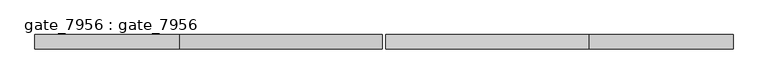
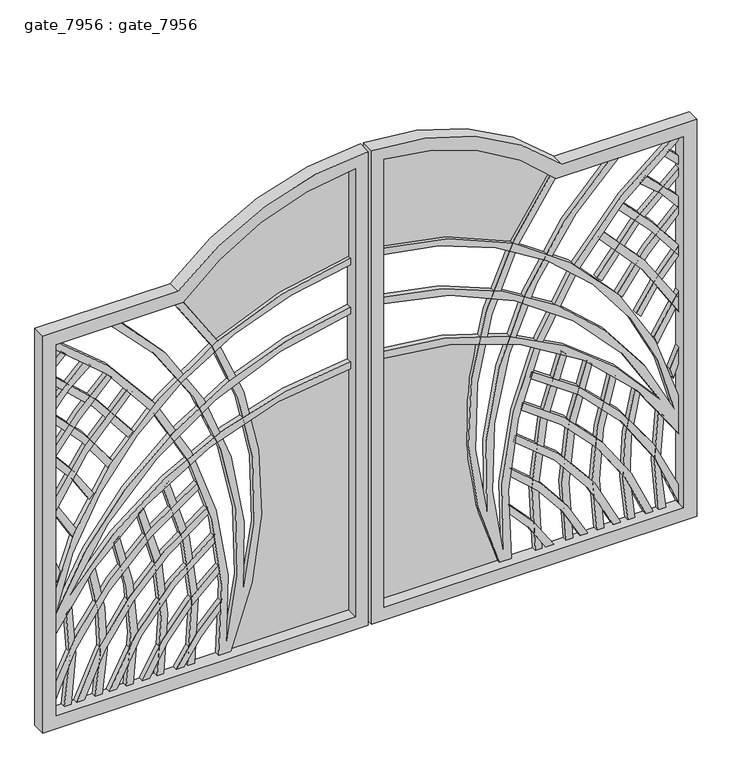
"""IFC4 building model written with IfcOpenShell, lengths in millimetres: proxy geometry, gate_7956 : gate_7956."""

from ifc_helpers import new_model, si_unit, point, frame, frame_2d, origin, place, context, project, spatial, polyline, circle_curve, trimmed, segment, composite_curve, outline, extrude, source, transform, mapped, element, save


def gate_7956_gate_7956_6bc30956(model_context):
    return source(origin(), model_context, "Body", "SweptSolid", [
        extrude(outline(composite_curve([segment(polyline([(1574.8, -714.375), (1574.8, -1222.375), (0.0, -1222.375), (0.0, 0.0), (1879.3736556, 0.0)]), True, "CONTINUOUS"), segment(trimmed(circle_curve(frame_2d((881.859553, 3.175)), 997.5191555), [point((1879.3736556, 0.0))], [point((1574.8, -714.375))], False, "CARTESIAN"), True, "CONTINUOUS")], self_intersect=False), holes=[composite_curve([segment(polyline([(1827.2147875, -47.625), (50.8, -47.625), (50.8, -1171.575), (1524.0, -1171.575), (1524.0, -692.4777911)]), True, "CONTINUOUS"), segment(trimmed(circle_curve(frame_2d((881.859553, 3.175)), 946.7191555), [point((1524.0, -692.4777911))], [point((1827.2147875, -47.625))], True, "CARTESIAN"), True, "CONTINUOUS")], self_intersect=False)]), frame((0.0, -50.8, 0.0), z_axis=(0.0, 1.0, 0.0), x_axis=(0.0, 0.0, 1.0)), (0.0, 0.0, 1.0), 50.8),
        extrude(outline(composite_curve([segment(trimmed(circle_curve(frame_2d((188.1193765, 65.6258097)), 1270.1981582), [point((1453.2587424, -47.625))], [point((475.7606767, -1171.575))], False, "CARTESIAN"), True, "CONTINUOUS"), segment(polyline([(475.7606767, -1171.575), (325.438753, -1171.575)]), True, "CONTINUOUS"), segment(trimmed(circle_curve(frame_2d((-306.470048, -9.2092819)), 1323.0278891), [point((325.438753, -1171.575))], [point((1016.0, -47.625))], True, "CARTESIAN"), True, "CONTINUOUS"), segment(polyline([(1016.0, -47.625), (1042.85139, -47.625)]), True, "CONTINUOUS"), segment(trimmed(circle_curve(frame_2d((-321.9912288, -1.7370637)), 1365.6138095), [point((1042.85139, -47.625))], [point((487.9033995, -1101.269586))], False, "CARTESIAN"), True, "CONTINUOUS"), segment(trimmed(circle_curve(frame_2d((-94.5667128, 101.7568292)), 1336.6166195), [point((487.9033995, -1101.269586))], [point((1233.6761327, -47.625))], True, "CARTESIAN"), True, "CONTINUOUS"), segment(polyline([(1233.6761327, -47.625), (1259.2332506, -47.625)]), True, "CONTINUOUS"), segment(trimmed(circle_curve(frame_2d((-94.5667128, 101.7568292)), 1362.0166195), [point((1259.2332506, -47.625))], [point((428.8390935, -1155.6753295))], False, "CARTESIAN"), True, "CONTINUOUS"), segment(trimmed(circle_curve(frame_2d((188.1193765, 65.6258097)), 1244.7981582), [point((428.8390935, -1155.6753295))], [point((1427.7550927, -47.625))], True, "CARTESIAN"), True, "CONTINUOUS"), segment(polyline([(1427.7550927, -47.625), (1453.2587424, -47.625)]), True, "CONTINUOUS")], self_intersect=False)), frame((0.0, -19.05, 0.0), z_axis=(0.0, 1.0, 0.0), x_axis=(0.0, 0.0, 1.0)), (0.0, 0.0, 1.0), 19.05),
        extrude(outline(composite_curve([segment(trimmed(circle_curve(frame_2d((625.1927136, -1831.8247988)), 1451.1947292), [point((50.8, -499.1436094))], [point((1524.0, -692.4777911))], False, "CARTESIAN"), True, "CONTINUOUS"), segment(polyline([(1524.0, -692.4777911), (1524.0, -717.8616311), (1508.2761961, -712.4096154)]), True, "CONTINUOUS"), segment(trimmed(circle_curve(frame_2d((625.2005352, -1831.8604357)), 1425.8305516), [point((1508.2761961, -712.4096154))], [point((270.5135839, -450.849962))], True, "CARTESIAN"), True, "CONTINUOUS"), segment(trimmed(circle_curve(frame_2d((428.9211986, -1911.4736244)), 1469.1883662), [point((270.5135839, -450.849962))], [point((1524.0, -932.0263955))], False, "CARTESIAN"), True, "CONTINUOUS"), segment(polyline([(1524.0, -932.0263955), (1524.0, -970.5462776)]), True, "CONTINUOUS"), segment(trimmed(circle_curve(frame_2d((434.6192112, -1905.6521568)), 1435.6787622), [point((1524.0, -970.5462776))], [point((79.5169904, -514.5820935))], True, "CARTESIAN"), True, "CONTINUOUS"), segment(trimmed(circle_curve(frame_2d((251.9754674, -2051.8469137)), 1546.9082241), [point((79.5169904, -514.5820935))], [point((1524.0, -1171.575))], False, "CARTESIAN"), True, "CONTINUOUS"), segment(polyline([(1524.0, -1171.575), (1492.986601, -1171.575)]), True, "CONTINUOUS"), segment(trimmed(circle_curve(frame_2d((251.9754674, -2051.8469137)), 1521.5082241), [point((1492.986601, -1171.575))], [point((50.8, -543.6971508))], True, "CARTESIAN"), True, "CONTINUOUS"), segment(polyline([(50.8, -543.6971508), (50.8, -499.1436094)]), True, "CONTINUOUS")], self_intersect=False)), frame((0.0, -19.05, 0.0), z_axis=(0.0, 1.0, 0.0), x_axis=(0.0, 0.0, 1.0)), (0.0, 0.0, 1.0), 19.05),
        extrude(outline(composite_curve([segment(trimmed(circle_curve(frame_2d((-321.9912288, -1.7370636)), 1251.3138095), [point((766.023996, -619.8059275))], [point((122.1545272, -1171.575))], False, "CARTESIAN"), True, "CONTINUOUS"), segment(polyline([(122.1545272, -1171.575), (50.8, -1171.575)]), True, "CONTINUOUS"), segment(trimmed(circle_curve(frame_2d((-329.3476454, 3.2021804)), 1234.7524675), [point((50.8, -1171.575))], [point((741.6413557, -611.2864))], True, "CARTESIAN"), True, "CONTINUOUS"), segment(polyline([(741.6413557, -611.2864), (766.023996, -619.8059275)]), True, "CONTINUOUS")], self_intersect=False)), frame((0.0, -19.05, 0.0), z_axis=(0.0, 1.0, 0.0), x_axis=(0.0, 0.0, 1.0)), (0.0, 0.0, 1.0), 19.05),
        extrude(outline(composite_curve([segment(trimmed(circle_curve(frame_2d((-321.9912288, -1.7370637)), 1137.0138095), [point((654.3216834, -584.5007383))], [point((50.8, -1075.9005069))], False, "CARTESIAN"), True, "CONTINUOUS"), segment(polyline([(50.8, -1075.9005069), (50.8, -1048.9772277)]), True, "CONTINUOUS"), segment(trimmed(circle_curve(frame_2d((-321.9912288, -1.7370637)), 1111.6138095), [point((50.8, -1048.9772277))], [point((628.7552213, -577.7287729))], True, "CARTESIAN"), True, "CONTINUOUS"), segment(polyline([(628.7552213, -577.7287729), (654.3216834, -584.5007383)]), True, "CONTINUOUS")], self_intersect=False)), frame((0.0, -19.05, 0.0), z_axis=(0.0, 1.0, 0.0), x_axis=(0.0, 0.0, 1.0)), (0.0, 0.0, 1.0), 19.05),
        extrude(outline(composite_curve([segment(trimmed(circle_curve(frame_2d((-321.9912288, -1.7370637)), 1022.7138095), [point((536.7182406, -557.2202617))], [point((50.8, -954.0869132))], False, "CARTESIAN"), True, "CONTINUOUS"), segment(polyline([(50.8, -954.0869132), (50.8, -926.7568118)]), True, "CONTINUOUS"), segment(trimmed(circle_curve(frame_2d((-321.9912288, -1.7370637)), 997.3138095), [point((50.8, -926.7568118))], [point((510.8571668, -550.3702604))], True, "CARTESIAN"), True, "CONTINUOUS"), segment(polyline([(510.8571668, -550.3702604), (536.7182406, -557.2202617)]), True, "CONTINUOUS")], self_intersect=False)), frame((0.0, -19.05, 0.0), z_axis=(0.0, 1.0, 0.0), x_axis=(0.0, 0.0, 1.0)), (0.0, 0.0, 1.0), 19.05),
        extrude(outline(composite_curve([segment(trimmed(circle_curve(frame_2d((-321.9912288, -1.7370637)), 908.4138095), [point((410.7722159, -538.6480277))], [point((50.8, -830.134522))], False, "CARTESIAN"), True, "CONTINUOUS"), segment(polyline([(50.8, -830.134522), (50.8, -802.1994847)]), True, "CONTINUOUS"), segment(trimmed(circle_curve(frame_2d((-321.9912288, -1.7370637)), 883.0138095), [point((50.8, -802.1994847))], [point((379.0365912, -538.6480277))], True, "CARTESIAN"), True, "CONTINUOUS"), segment(polyline([(379.0365912, -538.6480277), (410.7722159, -538.6480277)]), True, "CONTINUOUS")], self_intersect=False)), frame((0.0, -19.05, 0.0), z_axis=(0.0, 1.0, 0.0), x_axis=(0.0, 0.0, 1.0)), (0.0, 0.0, 1.0), 19.05),
        extrude(outline(composite_curve([segment(trimmed(circle_curve(frame_2d((-321.9912288, -1.7370637)), 794.1138095), [point((270.5266887, -530.4517881))], [point((50.8, -702.9099683))], False, "CARTESIAN"), True, "CONTINUOUS"), segment(polyline([(50.8, -702.9099683), (50.8, -674.0075603)]), True, "CONTINUOUS"), segment(trimmed(circle_curve(frame_2d((-321.9912288, -1.7370637)), 768.7138095), [point((50.8, -674.0075603))], [point((236.0245963, -530.4517881))], True, "CARTESIAN"), True, "CONTINUOUS"), segment(polyline([(236.0245963, -530.4517881), (270.5266887, -530.4517881)]), True, "CONTINUOUS")], self_intersect=False)), frame((0.0, -19.05, 0.0), z_axis=(0.0, 1.0, 0.0), x_axis=(0.0, 0.0, 1.0)), (0.0, 0.0, 1.0), 19.05),
        extrude(outline(composite_curve([segment(polyline([(1210.9602193, -867.4506933), (1228.939295, -885.429769)]), True, "CONTINUOUS"), segment(trimmed(circle_curve(frame_2d((188.1193765, 65.6258097)), 1409.8981582), [point((1228.939295, -885.429769))], [point((864.245824, -1171.575))], False, "CARTESIAN"), True, "CONTINUOUS"), segment(polyline([(864.245824, -1171.575), (809.5445985, -1171.575)]), True, "CONTINUOUS"), segment(trimmed(circle_curve(frame_2d((188.1193765, 65.6258097)), 1384.4981582), [point((809.5445985, -1171.575))], [point((1210.9602193, -867.4506933))], True, "CARTESIAN"), True, "CONTINUOUS")], self_intersect=False)), frame((0.0, -19.05, 0.0), z_axis=(0.0, 1.0, 0.0), x_axis=(0.0, 0.0, 1.0)), (0.0, 0.0, 1.0), 19.05),
        extrude(outline(composite_curve([segment(polyline([(1295.7670706, -944.0833092), (1313.7464656, -962.0627043)]), True, "CONTINUOUS"), segment(trimmed(circle_curve(frame_2d((298.9547736, -40.580869)), 1370.7410225), [point((1313.7464656, -962.0627043))], [point((1073.4115036, -1171.575))], False, "CARTESIAN"), True, "CONTINUOUS"), segment(polyline([(1073.4115036, -1171.575), (1034.1276953, -1171.575)]), True, "CONTINUOUS"), segment(trimmed(circle_curve(frame_2d((188.1193765, 65.6258097)), 1498.7981582), [point((1034.1276953, -1171.575))], [point((1295.7670706, -944.0833092))], True, "CARTESIAN"), True, "CONTINUOUS")], self_intersect=False)), frame((0.0, -19.05, 0.0), z_axis=(0.0, 1.0, 0.0), x_axis=(0.0, 0.0, 1.0)), (0.0, 0.0, 1.0), 19.05),
        extrude(outline(composite_curve([segment(polyline([(1371.3808408, -1023.8325474), (1393.8084123, -1046.2601189)]), True, "CONTINUOUS"), segment(trimmed(circle_curve(frame_2d((157.0059526, 65.2274597)), 1662.854462), [point((1393.8084123, -1046.2601189))], [point((1268.4935312, -1171.575))], False, "CARTESIAN"), True, "CONTINUOUS"), segment(polyline([(1268.4935312, -1171.575), (1223.2134903, -1171.575)]), True, "CONTINUOUS"), segment(trimmed(circle_curve(frame_2d((881.0604584, -680.2699964)), 598.7063586), [point((1223.2134903, -1171.575))], [point((1371.3808408, -1023.8325474))], True, "CARTESIAN"), True, "CONTINUOUS")], self_intersect=False)), frame((0.0, -19.05, 0.0), z_axis=(0.0, 1.0, 0.0), x_axis=(0.0, 0.0, 1.0)), (0.0, 0.0, 1.0), 19.05),
        extrude(outline(composite_curve([segment(polyline([(1448.1437026, -1116.942791), (1466.2607278, -1135.0598162)]), True, "CONTINUOUS"), segment(trimmed(circle_curve(frame_2d((2369.5144168, -2074.828689)), 1303.469509), [point((1466.2607278, -1135.0598162))], [point((1429.745544, -1171.575))], True, "CARTESIAN"), True, "CONTINUOUS"), segment(polyline([(1429.745544, -1171.575), (1393.6228205, -1171.575)]), True, "CONTINUOUS"), segment(trimmed(circle_curve(frame_2d((2581.8039176, -2302.8138821)), 1640.5717686), [point((1393.6228205, -1171.575))], [point((1448.1437026, -1116.942791))], False, "CARTESIAN"), True, "CONTINUOUS")], self_intersect=False)), frame((0.0, -19.05, 0.0), z_axis=(0.0, 1.0, 0.0), x_axis=(0.0, 0.0, 1.0)), (0.0, 0.0, 1.0), 19.05),
        extrude(outline(composite_curve([segment(polyline([(50.8, -1123.3836365), (50.8, -1096.2682984)]), True, "CONTINUOUS"), segment(trimmed(circle_curve(frame_2d((249.227799, -2294.693819)), 1214.741668), [point((50.8, -1096.2682984))], [point((439.2593722, -1094.9082877))], False, "CARTESIAN"), True, "CONTINUOUS"), segment(polyline([(439.2593722, -1094.9082877), (417.7529701, -1116.4146899)]), True, "CONTINUOUS"), segment(trimmed(circle_curve(frame_2d((251.9754674, -2051.8469137)), 950.0082241), [point((417.7529701, -1116.4146899))], [point((50.8, -1123.3836365))], True, "CARTESIAN"), True, "CONTINUOUS")], self_intersect=False)), frame((0.0, -19.05, 0.0), z_axis=(0.0, 1.0, 0.0), x_axis=(0.0, 0.0, 1.0)), (0.0, 0.0, 1.0), 19.05),
        extrude(outline(composite_curve([segment(polyline([(50.8, -1006.7247069), (50.8, -980.869582)]), True, "CONTINUOUS"), segment(trimmed(circle_curve(frame_2d((251.9754674, -2051.8469137)), 1089.7082241), [point((50.8, -980.869582))], [point((559.4182819, -1006.4078053))], False, "CARTESIAN"), True, "CONTINUOUS"), segment(polyline([(559.4182819, -1006.4078053), (538.8861292, -1026.939958)]), True, "CONTINUOUS"), segment(trimmed(circle_curve(frame_2d((251.9754674, -2051.8469137)), 1064.3082241), [point((538.8861292, -1026.939958))], [point((50.8, -1006.7247069))], True, "CARTESIAN"), True, "CONTINUOUS")], self_intersect=False)), frame((0.0, -19.05, 0.0), z_axis=(0.0, 1.0, 0.0), x_axis=(0.0, 0.0, 1.0)), (0.0, 0.0, 1.0), 19.05),
        extrude(outline(composite_curve([segment(polyline([(50.8, -890.30598), (50.8, -864.7646777)]), True, "CONTINUOUS"), segment(trimmed(circle_curve(frame_2d((251.9754674, -2051.8469137)), 1204.0082241), [point((50.8, -864.7646777))], [point((656.0575932, -917.6716895))], False, "CARTESIAN"), True, "CONTINUOUS"), segment(polyline([(656.0575932, -917.6716895), (636.1282841, -937.6009986)]), True, "CONTINUOUS"), segment(trimmed(circle_curve(frame_2d((249.671635, -2074.7397377)), 1201.0134277), [point((636.1282841, -937.6009986))], [point((50.8, -890.30598))], True, "CARTESIAN"), True, "CONTINUOUS")], self_intersect=False)), frame((0.0, -19.05, 0.0), z_axis=(0.0, 1.0, 0.0), x_axis=(0.0, 0.0, 1.0)), (0.0, 0.0, 1.0), 19.05),
        extrude(outline(composite_curve([segment(polyline([(50.8, -774.6859578), (50.8, -748.9789216)]), True, "CONTINUOUS"), segment(trimmed(circle_curve(frame_2d((251.9754674, -2051.8469137)), 1318.3082241), [point((50.8, -748.9789216))], [point((737.9350335, -826.3756274))], False, "CARTESIAN"), True, "CONTINUOUS"), segment(polyline([(737.9350335, -826.3756274), (718.3335001, -845.9771607)]), True, "CONTINUOUS"), segment(trimmed(circle_curve(frame_2d((251.9754674, -2051.8469137)), 1292.9082241), [point((718.3335001, -845.9771607))], [point((50.8, -774.6859578))], True, "CARTESIAN"), True, "CONTINUOUS")], self_intersect=False)), frame((0.0, -19.05, 0.0), z_axis=(0.0, 1.0, 0.0), x_axis=(0.0, 0.0, 1.0)), (0.0, 0.0, 1.0), 19.05),
        extrude(outline(composite_curve([segment(polyline([(50.8, -659.0930168), (50.8, -633.4341547)]), True, "CONTINUOUS"), segment(trimmed(circle_curve(frame_2d((251.9754674, -2051.8469137)), 1432.6082241), [point((50.8, -633.4341547))], [point((808.380048, -731.7028813))], False, "CARTESIAN"), True, "CONTINUOUS"), segment(polyline([(808.380048, -731.7028813), (788.9599222, -751.1230071)]), True, "CONTINUOUS"), segment(trimmed(circle_curve(frame_2d((251.9754674, -2051.8469137)), 1407.2082241), [point((788.9599222, -751.1230071))], [point((50.8, -659.0930168))], True, "CARTESIAN"), True, "CONTINUOUS")], self_intersect=False)), frame((0.0, -19.05, 0.0), z_axis=(0.0, 1.0, 0.0), x_axis=(0.0, 0.0, 1.0)), (0.0, 0.0, 1.0), 19.05),
        extrude(outline(polyline([(553.3842288, -1150.9205103), (593.450224, -1138.1641492), (672.1451492, -1171.575), (609.2386529, -1171.575), (553.3842288, -1150.9205103)])), frame((0.0, -19.05, 0.0), z_axis=(0.0, 1.0, 0.0), x_axis=(0.0, 0.0, 1.0)), (0.0, 0.0, 1.0), 19.05),
        extrude(outline(composite_curve([segment(trimmed(circle_curve(frame_2d((251.9754673, -2051.8469137)), 1064.3082241), [point((850.2006371, -1171.575))], [point((711.3700205, -1091.7903318))], True, "CARTESIAN"), True, "CONTINUOUS"), segment(polyline([(711.3700205, -1091.7903318), (740.9012216, -1077.980588)]), True, "CONTINUOUS"), segment(trimmed(circle_curve(frame_2d((251.9754674, -2051.8469137)), 1089.7082241), [point((740.9012216, -1077.980588))], [point((894.3035545, -1171.575))], False, "CARTESIAN"), True, "CONTINUOUS"), segment(polyline([(894.3035545, -1171.575), (850.2006371, -1171.575)]), True, "CONTINUOUS")], self_intersect=False)), frame((0.0, -19.05, 0.0), z_axis=(0.0, 1.0, 0.0), x_axis=(0.0, 0.0, 1.0)), (0.0, 0.0, 1.0), 19.05),
        extrude(outline(composite_curve([segment(trimmed(circle_curve(frame_2d((436.5150762, -1780.3292563)), 853.0665783), [point((1034.1276953, -1171.575))], [point((842.2813497, -1029.9451424))], True, "CARTESIAN"), True, "CONTINUOUS"), segment(polyline([(842.2813497, -1029.9451424), (859.7363544, -1012.4901377)]), True, "CONTINUOUS"), segment(trimmed(circle_curve(frame_2d((251.9754673, -2051.8469137)), 1204.0082241), [point((859.7363544, -1012.4901377))], [point((1073.4115036, -1171.575))], False, "CARTESIAN"), True, "CONTINUOUS"), segment(polyline([(1073.4115036, -1171.575), (1034.1276953, -1171.575)]), True, "CONTINUOUS")], self_intersect=False)), frame((0.0, -19.05, 0.0), z_axis=(0.0, 1.0, 0.0), x_axis=(0.0, 0.0, 1.0)), (0.0, 0.0, 1.0), 19.05),
        extrude(outline(composite_curve([segment(polyline([(943.9740273, -959.7161207), (962.3717805, -941.3183675)]), True, "CONTINUOUS"), segment(trimmed(circle_curve(frame_2d((251.9754673, -2051.8469138)), 1318.3082242), [point((962.3717805, -941.3183675))], [point((1233.3306179, -1171.575))], False, "CARTESIAN"), True, "CONTINUOUS"), segment(polyline([(1233.3306179, -1171.575), (1198.9353576, -1171.575)]), True, "CONTINUOUS"), segment(trimmed(circle_curve(frame_2d((251.9754673, -2051.8469138)), 1292.9082241), [point((1198.9353576, -1171.575))], [point((943.9740273, -959.7161207))], True, "CARTESIAN"), True, "CONTINUOUS")], self_intersect=False)), frame((0.0, -19.05, 0.0), z_axis=(0.0, 1.0, 0.0), x_axis=(0.0, 0.0, 1.0)), (0.0, 0.0, 1.0), 19.05),
        extrude(outline(composite_curve([segment(polyline([(1035.0267606, -882.6310833), (1053.3289179, -864.3289261)]), True, "CONTINUOUS"), segment(trimmed(circle_curve(frame_2d((251.9754673, -2051.8469137)), 1432.6082241), [point((1053.3289179, -864.3289261))], [point((1382.2354736, -1171.575))], False, "CARTESIAN"), True, "CONTINUOUS"), segment(polyline([(1382.2354736, -1171.575), (1349.8626855, -1171.575)]), True, "CONTINUOUS"), segment(trimmed(circle_curve(frame_2d((251.9754674, -2051.8469137)), 1407.2082241), [point((1349.8626855, -1171.575))], [point((1035.0267606, -882.6310833))], True, "CARTESIAN"), True, "CONTINUOUS")], self_intersect=False)), frame((0.0, -19.05, 0.0), z_axis=(0.0, 1.0, 0.0), x_axis=(0.0, 0.0, 1.0)), (0.0, 0.0, 1.0), 19.05),
        extrude(outline(composite_curve([segment(trimmed(circle_curve(frame_2d((881.859553, 3.175)), 946.7191555), [point((1827.2147875, -47.625))], [point((1524.0, -692.4777911))], False, "CARTESIAN"), True, "CONTINUOUS"), segment(trimmed(circle_curve(frame_2d((625.1927137, -1831.8247988)), 1451.1947292), [point((1524.0, -692.4777911))], [point((1300.6036994, -547.3847876))], True, "CARTESIAN"), True, "CONTINUOUS"), segment(trimmed(circle_curve(frame_2d((188.1193765, 65.6258097)), 1270.1981582), [point((1300.6036994, -547.3847876))], [point((1453.2587424, -47.625))], True, "CARTESIAN"), True, "CONTINUOUS"), segment(polyline([(1453.2587424, -47.625), (1827.2147875, -47.625)]), True, "CONTINUOUS")], self_intersect=False)), frame((0.0, -6.35, 0.0), z_axis=(0.0, 1.0, 0.0), x_axis=(0.0, 0.0, 1.0)), (0.0, 0.0, 1.0), 6.35),
        extrude(outline(composite_curve([segment(trimmed(circle_curve(frame_2d((-306.470048, -9.2092819)), 1323.0278891), [point((1016.0, -47.625))], [point((951.8602911, -417.8748577))], False, "CARTESIAN"), True, "CONTINUOUS"), segment(trimmed(circle_curve(frame_2d((625.1927136, -1831.8247988)), 1451.1947292), [point((951.8602911, -417.8748577))], [point((50.8, -499.1436094))], True, "CARTESIAN"), True, "CONTINUOUS"), segment(polyline([(50.8, -499.1436094), (50.8, -47.625), (1016.0, -47.625)]), True, "CONTINUOUS")], self_intersect=False)), frame((0.0, -6.35, 0.0), z_axis=(0.0, 1.0, 0.0), x_axis=(0.0, 0.0, 1.0)), (0.0, 0.0, 1.0), 6.35),
        extrude(outline(composite_curve([segment(trimmed(circle_curve(frame_2d((881.859553, 9.525)), 997.5191555), [point((1574.8, 727.075))], [point((1879.3736556, 12.7))], False, "CARTESIAN"), True, "CONTINUOUS"), segment(polyline([(1879.3736556, 12.7), (0.0, 12.7), (0.0, 1235.075), (1574.8, 1235.075), (1574.8, 727.075)]), True, "CONTINUOUS")], self_intersect=False), holes=[composite_curve([segment(trimmed(circle_curve(frame_2d((881.859553, 9.525)), 946.7191555), [point((1827.2147875, 60.325))], [point((1524.0, 705.1777911))], True, "CARTESIAN"), True, "CONTINUOUS"), segment(polyline([(1524.0, 705.1777911), (1524.0, 1184.275), (50.8, 1184.275), (50.8, 60.325), (1827.2147875, 60.325)]), True, "CONTINUOUS")], self_intersect=False)]), frame((0.0, -50.8, 0.0), z_axis=(0.0, 1.0, 0.0), x_axis=(0.0, 0.0, 1.0)), (0.0, 0.0, 1.0), 50.8),
        extrude(outline(composite_curve([segment(polyline([(1453.2587424, 60.325), (1427.7550927, 60.325)]), True, "CONTINUOUS"), segment(trimmed(circle_curve(frame_2d((188.1193765, -52.9258097)), 1244.7981582), [point((1427.7550927, 60.325))], [point((428.8390935, 1168.3753295))], True, "CARTESIAN"), True, "CONTINUOUS"), segment(trimmed(circle_curve(frame_2d((-94.5667128, -89.0568292)), 1362.0166195), [point((428.8390935, 1168.3753295))], [point((1259.2332506, 60.325))], False, "CARTESIAN"), True, "CONTINUOUS"), segment(polyline([(1259.2332506, 60.325), (1233.6761327, 60.325)]), True, "CONTINUOUS"), segment(trimmed(circle_curve(frame_2d((-94.5667128, -89.0568292)), 1336.6166195), [point((1233.6761327, 60.325))], [point((487.9033995, 1113.969586))], True, "CARTESIAN"), True, "CONTINUOUS"), segment(trimmed(circle_curve(frame_2d((-321.9912288, 14.4370637)), 1365.6138095), [point((487.9033995, 1113.969586))], [point((1042.85139, 60.325))], False, "CARTESIAN"), True, "CONTINUOUS"), segment(polyline([(1042.85139, 60.325), (1016.0, 60.325)]), True, "CONTINUOUS"), segment(trimmed(circle_curve(frame_2d((-306.470048, 21.9092819)), 1323.0278891), [point((1016.0, 60.325))], [point((325.438753, 1184.275))], True, "CARTESIAN"), True, "CONTINUOUS"), segment(polyline([(325.438753, 1184.275), (475.7606767, 1184.275)]), True, "CONTINUOUS"), segment(trimmed(circle_curve(frame_2d((188.1193765, -52.9258097)), 1270.1981582), [point((475.7606767, 1184.275))], [point((1453.2587424, 60.325))], False, "CARTESIAN"), True, "CONTINUOUS")], self_intersect=False)), frame((0.0, -19.05, 0.0), z_axis=(0.0, 1.0, 0.0), x_axis=(0.0, 0.0, 1.0)), (0.0, 0.0, 1.0), 19.05),
        extrude(outline(composite_curve([segment(polyline([(50.8, 511.8436094), (50.8, 556.3971508)]), True, "CONTINUOUS"), segment(trimmed(circle_curve(frame_2d((251.9754674, 2064.5469137)), 1521.5082241), [point((50.8, 556.3971508))], [point((1492.986601, 1184.275))], True, "CARTESIAN"), True, "CONTINUOUS"), segment(polyline([(1492.986601, 1184.275), (1524.0, 1184.275)]), True, "CONTINUOUS"), segment(trimmed(circle_curve(frame_2d((251.9754674, 2064.5469137)), 1546.9082241), [point((1524.0, 1184.275))], [point((79.5169904, 527.2820935))], False, "CARTESIAN"), True, "CONTINUOUS"), segment(trimmed(circle_curve(frame_2d((434.6192112, 1918.3521568)), 1435.6787622), [point((79.5169904, 527.2820935))], [point((1524.0, 983.2462776))], True, "CARTESIAN"), True, "CONTINUOUS"), segment(polyline([(1524.0, 983.2462776), (1524.0, 944.7263955)]), True, "CONTINUOUS"), segment(trimmed(circle_curve(frame_2d((428.9211986, 1924.1736244)), 1469.1883662), [point((1524.0, 944.7263955))], [point((270.5135839, 463.549962))], False, "CARTESIAN"), True, "CONTINUOUS"), segment(trimmed(circle_curve(frame_2d((625.2005352, 1844.5604357)), 1425.8305516), [point((270.5135839, 463.549962))], [point((1508.2761961, 725.1096154))], True, "CARTESIAN"), True, "CONTINUOUS"), segment(polyline([(1508.2761961, 725.1096154), (1524.0, 730.5616311), (1524.0, 705.1777911)]), True, "CONTINUOUS"), segment(trimmed(circle_curve(frame_2d((625.1927136, 1844.5247988)), 1451.1947292), [point((1524.0, 705.1777911))], [point((50.8, 511.8436094))], False, "CARTESIAN"), True, "CONTINUOUS")], self_intersect=False)), frame((0.0, -19.05, 0.0), z_axis=(0.0, 1.0, 0.0), x_axis=(0.0, 0.0, 1.0)), (0.0, 0.0, 1.0), 19.05),
        extrude(outline(composite_curve([segment(polyline([(766.023996, 632.5059275), (741.6413557, 623.9864)]), True, "CONTINUOUS"), segment(trimmed(circle_curve(frame_2d((-329.3476454, 9.4978196)), 1234.7524675), [point((741.6413557, 623.9864))], [point((50.8, 1184.275))], True, "CARTESIAN"), True, "CONTINUOUS"), segment(polyline([(50.8, 1184.275), (122.1545272, 1184.275)]), True, "CONTINUOUS"), segment(trimmed(circle_curve(frame_2d((-321.9912288, 14.4370636)), 1251.3138095), [point((122.1545272, 1184.275))], [point((766.023996, 632.5059275))], False, "CARTESIAN"), True, "CONTINUOUS")], self_intersect=False)), frame((0.0, -19.05, 0.0), z_axis=(0.0, 1.0, 0.0), x_axis=(0.0, 0.0, 1.0)), (0.0, 0.0, 1.0), 19.05),
        extrude(outline(composite_curve([segment(polyline([(654.3216834, 597.2007383), (628.7552213, 590.4287729)]), True, "CONTINUOUS"), segment(trimmed(circle_curve(frame_2d((-321.9912288, 14.4370637)), 1111.6138095), [point((628.7552213, 590.4287729))], [point((50.8, 1061.6772277))], True, "CARTESIAN"), True, "CONTINUOUS"), segment(polyline([(50.8, 1061.6772277), (50.8, 1088.6005069)]), True, "CONTINUOUS"), segment(trimmed(circle_curve(frame_2d((-321.9912288, 14.4370637)), 1137.0138095), [point((50.8, 1088.6005069))], [point((654.3216834, 597.2007383))], False, "CARTESIAN"), True, "CONTINUOUS")], self_intersect=False)), frame((0.0, -19.05, 0.0), z_axis=(0.0, 1.0, 0.0), x_axis=(0.0, 0.0, 1.0)), (0.0, 0.0, 1.0), 19.05),
        extrude(outline(composite_curve([segment(polyline([(536.7182406, 569.9202617), (510.8571668, 563.0702604)]), True, "CONTINUOUS"), segment(trimmed(circle_curve(frame_2d((-321.9912288, 14.4370637)), 997.3138095), [point((510.8571668, 563.0702604))], [point((50.8, 939.4568118))], True, "CARTESIAN"), True, "CONTINUOUS"), segment(polyline([(50.8, 939.4568118), (50.8, 966.7869132)]), True, "CONTINUOUS"), segment(trimmed(circle_curve(frame_2d((-321.9912288, 14.4370637)), 1022.7138095), [point((50.8, 966.7869132))], [point((536.7182406, 569.9202617))], False, "CARTESIAN"), True, "CONTINUOUS")], self_intersect=False)), frame((0.0, -19.05, 0.0), z_axis=(0.0, 1.0, 0.0), x_axis=(0.0, 0.0, 1.0)), (0.0, 0.0, 1.0), 19.05),
        extrude(outline(composite_curve([segment(polyline([(410.7722159, 551.3480277), (379.0365912, 551.3480277)]), True, "CONTINUOUS"), segment(trimmed(circle_curve(frame_2d((-321.9912288, 14.4370637)), 883.0138095), [point((379.0365912, 551.3480277))], [point((50.8, 814.8994847))], True, "CARTESIAN"), True, "CONTINUOUS"), segment(polyline([(50.8, 814.8994847), (50.8, 842.834522)]), True, "CONTINUOUS"), segment(trimmed(circle_curve(frame_2d((-321.9912288, 14.4370637)), 908.4138095), [point((50.8, 842.834522))], [point((410.7722159, 551.3480277))], False, "CARTESIAN"), True, "CONTINUOUS")], self_intersect=False)), frame((0.0, -19.05, 0.0), z_axis=(0.0, 1.0, 0.0), x_axis=(0.0, 0.0, 1.0)), (0.0, 0.0, 1.0), 19.05),
        extrude(outline(composite_curve([segment(polyline([(270.5266887, 543.1517881), (236.0245963, 543.1517881)]), True, "CONTINUOUS"), segment(trimmed(circle_curve(frame_2d((-321.9912288, 14.4370637)), 768.7138095), [point((236.0245963, 543.1517881))], [point((50.8, 686.7075603))], True, "CARTESIAN"), True, "CONTINUOUS"), segment(polyline([(50.8, 686.7075603), (50.8, 715.6099683)]), True, "CONTINUOUS"), segment(trimmed(circle_curve(frame_2d((-321.9912288, 14.4370637)), 794.1138095), [point((50.8, 715.6099683))], [point((270.5266887, 543.1517881))], False, "CARTESIAN"), True, "CONTINUOUS")], self_intersect=False)), frame((0.0, -19.05, 0.0), z_axis=(0.0, 1.0, 0.0), x_axis=(0.0, 0.0, 1.0)), (0.0, 0.0, 1.0), 19.05),
        extrude(outline(composite_curve([segment(trimmed(circle_curve(frame_2d((188.1193765, -52.9258097)), 1384.4981582), [point((1210.9602193, 880.1506933))], [point((809.5445985, 1184.275))], True, "CARTESIAN"), True, "CONTINUOUS"), segment(polyline([(809.5445985, 1184.275), (864.245824, 1184.275)]), True, "CONTINUOUS"), segment(trimmed(circle_curve(frame_2d((188.1193765, -52.9258097)), 1409.8981582), [point((864.245824, 1184.275))], [point((1228.939295, 898.129769))], False, "CARTESIAN"), True, "CONTINUOUS"), segment(polyline([(1228.939295, 898.129769), (1210.9602193, 880.1506933)]), True, "CONTINUOUS")], self_intersect=False)), frame((0.0, -19.05, 0.0), z_axis=(0.0, 1.0, 0.0), x_axis=(0.0, 0.0, 1.0)), (0.0, 0.0, 1.0), 19.05),
        extrude(outline(composite_curve([segment(trimmed(circle_curve(frame_2d((188.1193765, -52.9258097)), 1498.7981582), [point((1295.7670706, 956.7833092))], [point((1034.1276953, 1184.275))], True, "CARTESIAN"), True, "CONTINUOUS"), segment(polyline([(1034.1276953, 1184.275), (1073.4115036, 1184.275)]), True, "CONTINUOUS"), segment(trimmed(circle_curve(frame_2d((298.9547736, 53.280869)), 1370.7410225), [point((1073.4115036, 1184.275))], [point((1313.7464656, 974.7627043))], False, "CARTESIAN"), True, "CONTINUOUS"), segment(polyline([(1313.7464656, 974.7627043), (1295.7670706, 956.7833092)]), True, "CONTINUOUS")], self_intersect=False)), frame((0.0, -19.05, 0.0), z_axis=(0.0, 1.0, 0.0), x_axis=(0.0, 0.0, 1.0)), (0.0, 0.0, 1.0), 19.05),
        extrude(outline(composite_curve([segment(trimmed(circle_curve(frame_2d((881.0604584, 692.9699964)), 598.7063586), [point((1371.3808408, 1036.5325474))], [point((1223.2134903, 1184.275))], True, "CARTESIAN"), True, "CONTINUOUS"), segment(polyline([(1223.2134903, 1184.275), (1268.4935312, 1184.275)]), True, "CONTINUOUS"), segment(trimmed(circle_curve(frame_2d((157.0059526, -52.5274597)), 1662.854462), [point((1268.4935312, 1184.275))], [point((1393.8084123, 1058.9601189))], False, "CARTESIAN"), True, "CONTINUOUS"), segment(polyline([(1393.8084123, 1058.9601189), (1371.3808408, 1036.5325474)]), True, "CONTINUOUS")], self_intersect=False)), frame((0.0, -19.05, 0.0), z_axis=(0.0, 1.0, 0.0), x_axis=(0.0, 0.0, 1.0)), (0.0, 0.0, 1.0), 19.05),
        extrude(outline(composite_curve([segment(trimmed(circle_curve(frame_2d((2581.8039176, 2315.5138821)), 1640.5717686), [point((1448.1437026, 1129.642791))], [point((1393.6228205, 1184.275))], False, "CARTESIAN"), True, "CONTINUOUS"), segment(polyline([(1393.6228205, 1184.275), (1429.745544, 1184.275)]), True, "CONTINUOUS"), segment(trimmed(circle_curve(frame_2d((2369.5144168, 2087.528689)), 1303.469509), [point((1429.745544, 1184.275))], [point((1466.2607278, 1147.7598162))], True, "CARTESIAN"), True, "CONTINUOUS"), segment(polyline([(1466.2607278, 1147.7598162), (1448.1437026, 1129.642791)]), True, "CONTINUOUS")], self_intersect=False)), frame((0.0, -19.05, 0.0), z_axis=(0.0, 1.0, 0.0), x_axis=(0.0, 0.0, 1.0)), (0.0, 0.0, 1.0), 19.05),
        extrude(outline(composite_curve([segment(trimmed(circle_curve(frame_2d((251.9754674, 2064.5469137)), 950.0082241), [point((50.8, 1136.0836365))], [point((417.7529701, 1129.1146899))], True, "CARTESIAN"), True, "CONTINUOUS"), segment(polyline([(417.7529701, 1129.1146899), (439.2593722, 1107.6082877)]), True, "CONTINUOUS"), segment(trimmed(circle_curve(frame_2d((249.227799, 2307.393819)), 1214.741668), [point((439.2593722, 1107.6082877))], [point((50.8, 1108.9682984))], False, "CARTESIAN"), True, "CONTINUOUS"), segment(polyline([(50.8, 1108.9682984), (50.8, 1136.0836365)]), True, "CONTINUOUS")], self_intersect=False)), frame((0.0, -19.05, 0.0), z_axis=(0.0, 1.0, 0.0), x_axis=(0.0, 0.0, 1.0)), (0.0, 0.0, 1.0), 19.05),
        extrude(outline(composite_curve([segment(trimmed(circle_curve(frame_2d((251.9754674, 2064.5469137)), 1064.3082241), [point((50.8, 1019.4247069))], [point((538.8861292, 1039.639958))], True, "CARTESIAN"), True, "CONTINUOUS"), segment(polyline([(538.8861292, 1039.639958), (559.4182819, 1019.1078053)]), True, "CONTINUOUS"), segment(trimmed(circle_curve(frame_2d((251.9754674, 2064.5469137)), 1089.7082241), [point((559.4182819, 1019.1078053))], [point((50.8, 993.569582))], False, "CARTESIAN"), True, "CONTINUOUS"), segment(polyline([(50.8, 993.569582), (50.8, 1019.4247069)]), True, "CONTINUOUS")], self_intersect=False)), frame((0.0, -19.05, 0.0), z_axis=(0.0, 1.0, 0.0), x_axis=(0.0, 0.0, 1.0)), (0.0, 0.0, 1.0), 19.05),
        extrude(outline(composite_curve([segment(trimmed(circle_curve(frame_2d((249.671635, 2087.4397377)), 1201.0134277), [point((50.8, 903.00598))], [point((636.1282841, 950.3009986))], True, "CARTESIAN"), True, "CONTINUOUS"), segment(polyline([(636.1282841, 950.3009986), (656.0575932, 930.3716895)]), True, "CONTINUOUS"), segment(trimmed(circle_curve(frame_2d((251.9754674, 2064.5469137)), 1204.0082241), [point((656.0575932, 930.3716895))], [point((50.8, 877.4646777))], False, "CARTESIAN"), True, "CONTINUOUS"), segment(polyline([(50.8, 877.4646777), (50.8, 903.00598)]), True, "CONTINUOUS")], self_intersect=False)), frame((0.0, -19.05, 0.0), z_axis=(0.0, 1.0, 0.0), x_axis=(0.0, 0.0, 1.0)), (0.0, 0.0, 1.0), 19.05),
        extrude(outline(composite_curve([segment(trimmed(circle_curve(frame_2d((251.9754674, 2064.5469137)), 1292.9082241), [point((50.8, 787.3859578))], [point((718.3335001, 858.6771607))], True, "CARTESIAN"), True, "CONTINUOUS"), segment(polyline([(718.3335001, 858.6771607), (737.9350335, 839.0756274)]), True, "CONTINUOUS"), segment(trimmed(circle_curve(frame_2d((251.9754674, 2064.5469137)), 1318.3082241), [point((737.9350335, 839.0756274))], [point((50.8, 761.6789216))], False, "CARTESIAN"), True, "CONTINUOUS"), segment(polyline([(50.8, 761.6789216), (50.8, 787.3859578)]), True, "CONTINUOUS")], self_intersect=False)), frame((0.0, -19.05, 0.0), z_axis=(0.0, 1.0, 0.0), x_axis=(0.0, 0.0, 1.0)), (0.0, 0.0, 1.0), 19.05),
        extrude(outline(composite_curve([segment(trimmed(circle_curve(frame_2d((251.9754674, 2064.5469137)), 1407.2082241), [point((50.8, 671.7930168))], [point((788.9599222, 763.8230071))], True, "CARTESIAN"), True, "CONTINUOUS"), segment(polyline([(788.9599222, 763.8230071), (808.380048, 744.4028813)]), True, "CONTINUOUS"), segment(trimmed(circle_curve(frame_2d((251.9754674, 2064.5469137)), 1432.6082241), [point((808.380048, 744.4028813))], [point((50.8, 646.1341547))], False, "CARTESIAN"), True, "CONTINUOUS"), segment(polyline([(50.8, 646.1341547), (50.8, 671.7930168)]), True, "CONTINUOUS")], self_intersect=False)), frame((0.0, -19.05, 0.0), z_axis=(0.0, 1.0, 0.0), x_axis=(0.0, 0.0, 1.0)), (0.0, 0.0, 1.0), 19.05),
        extrude(outline(polyline([(553.3842288, 1163.6205103), (609.2386529, 1184.275), (672.1451492, 1184.275), (593.450224, 1150.8641492), (553.3842288, 1163.6205103)])), frame((0.0, -19.05, 0.0), z_axis=(0.0, 1.0, 0.0), x_axis=(0.0, 0.0, 1.0)), (0.0, 0.0, 1.0), 19.05),
        extrude(outline(composite_curve([segment(polyline([(850.2006371, 1184.275), (894.3035545, 1184.275)]), True, "CONTINUOUS"), segment(trimmed(circle_curve(frame_2d((251.9754674, 2064.5469137)), 1089.7082241), [point((894.3035545, 1184.275))], [point((740.9012216, 1090.680588))], False, "CARTESIAN"), True, "CONTINUOUS"), segment(polyline([(740.9012216, 1090.680588), (711.3700205, 1104.4903318)]), True, "CONTINUOUS"), segment(trimmed(circle_curve(frame_2d((251.9754673, 2064.5469137)), 1064.3082241), [point((711.3700205, 1104.4903318))], [point((850.2006371, 1184.275))], True, "CARTESIAN"), True, "CONTINUOUS")], self_intersect=False)), frame((0.0, -19.05, 0.0), z_axis=(0.0, 1.0, 0.0), x_axis=(0.0, 0.0, 1.0)), (0.0, 0.0, 1.0), 19.05),
        extrude(outline(composite_curve([segment(polyline([(1034.1276953, 1184.275), (1073.4115036, 1184.275)]), True, "CONTINUOUS"), segment(trimmed(circle_curve(frame_2d((251.9754673, 2064.5469137)), 1204.0082241), [point((1073.4115036, 1184.275))], [point((859.7363544, 1025.1901377))], False, "CARTESIAN"), True, "CONTINUOUS"), segment(polyline([(859.7363544, 1025.1901377), (842.2813497, 1042.6451424)]), True, "CONTINUOUS"), segment(trimmed(circle_curve(frame_2d((436.5150762, 1793.0292563)), 853.0665783), [point((842.2813497, 1042.6451424))], [point((1034.1276953, 1184.275))], True, "CARTESIAN"), True, "CONTINUOUS")], self_intersect=False)), frame((0.0, -19.05, 0.0), z_axis=(0.0, 1.0, 0.0), x_axis=(0.0, 0.0, 1.0)), (0.0, 0.0, 1.0), 19.05),
        extrude(outline(composite_curve([segment(trimmed(circle_curve(frame_2d((251.9754673, 2064.5469138)), 1292.9082241), [point((943.9740273, 972.4161207))], [point((1198.9353576, 1184.275))], True, "CARTESIAN"), True, "CONTINUOUS"), segment(polyline([(1198.9353576, 1184.275), (1233.3306179, 1184.275)]), True, "CONTINUOUS"), segment(trimmed(circle_curve(frame_2d((251.9754673, 2064.5469138)), 1318.3082242), [point((1233.3306179, 1184.275))], [point((962.3717805, 954.0183675))], False, "CARTESIAN"), True, "CONTINUOUS"), segment(polyline([(962.3717805, 954.0183675), (943.9740273, 972.4161207)]), True, "CONTINUOUS")], self_intersect=False)), frame((0.0, -19.05, 0.0), z_axis=(0.0, 1.0, 0.0), x_axis=(0.0, 0.0, 1.0)), (0.0, 0.0, 1.0), 19.05),
        extrude(outline(composite_curve([segment(trimmed(circle_curve(frame_2d((251.9754674, 2064.5469137)), 1407.2082241), [point((1035.0267606, 895.3310833))], [point((1349.8626855, 1184.275))], True, "CARTESIAN"), True, "CONTINUOUS"), segment(polyline([(1349.8626855, 1184.275), (1382.2354736, 1184.275)]), True, "CONTINUOUS"), segment(trimmed(circle_curve(frame_2d((251.9754673, 2064.5469137)), 1432.6082241), [point((1382.2354736, 1184.275))], [point((1053.3289179, 877.0289261))], False, "CARTESIAN"), True, "CONTINUOUS"), segment(polyline([(1053.3289179, 877.0289261), (1035.0267606, 895.3310833)]), True, "CONTINUOUS")], self_intersect=False)), frame((0.0, -19.05, 0.0), z_axis=(0.0, 1.0, 0.0), x_axis=(0.0, 0.0, 1.0)), (0.0, 0.0, 1.0), 19.05),
        extrude(outline(composite_curve([segment(polyline([(1827.2147875, 60.325), (1453.2587424, 60.325)]), True, "CONTINUOUS"), segment(trimmed(circle_curve(frame_2d((188.1193765, -52.9258097)), 1270.1981582), [point((1453.2587424, 60.325))], [point((1300.6036994, 560.0847876))], True, "CARTESIAN"), True, "CONTINUOUS"), segment(trimmed(circle_curve(frame_2d((625.1927137, 1844.5247988)), 1451.1947292), [point((1300.6036994, 560.0847876))], [point((1524.0, 705.1777911))], True, "CARTESIAN"), True, "CONTINUOUS"), segment(trimmed(circle_curve(frame_2d((881.859553, 9.525)), 946.7191555), [point((1524.0, 705.1777911))], [point((1827.2147875, 60.325))], False, "CARTESIAN"), True, "CONTINUOUS")], self_intersect=False)), frame((0.0, -6.35, 0.0), z_axis=(0.0, 1.0, 0.0), x_axis=(0.0, 0.0, 1.0)), (0.0, 0.0, 1.0), 6.35),
        extrude(outline(composite_curve([segment(polyline([(1016.0, 60.325), (50.8, 60.325), (50.8, 511.8436094)]), True, "CONTINUOUS"), segment(trimmed(circle_curve(frame_2d((625.1927136, 1844.5247988)), 1451.1947292), [point((50.8, 511.8436094))], [point((951.8602911, 430.5748577))], True, "CARTESIAN"), True, "CONTINUOUS"), segment(trimmed(circle_curve(frame_2d((-306.470048, 21.9092819)), 1323.0278891), [point((951.8602911, 430.5748577))], [point((1016.0, 60.325))], False, "CARTESIAN"), True, "CONTINUOUS")], self_intersect=False)), frame((0.0, -6.35, 0.0), z_axis=(0.0, 1.0, 0.0), x_axis=(0.0, 0.0, 1.0)), (0.0, 0.0, 1.0), 6.35),
    ])


if __name__ == "__main__":
    model = new_model("IFC4")
    model_context = context("Model", 3, world=origin())
    ifc_project = project(units=[si_unit("LENGTHUNIT", "METRE", prefix="MILLI")], contexts=[model_context])
    site = spatial("IfcSite", under=ifc_project)
    building = spatial("IfcBuilding", under=site)
    placement = place(None, origin())
    gate_7956_gate_7956_shape = gate_7956_gate_7956_6bc30956(model_context)
    element("IfcBuildingElementProxy", 1, Name="gate_7956 : gate_7956", ObjectType="gate_7956 : gate_7956", at=placement, inside=building, context=model_context, shape_type="MappedRepresentation", body=[
        mapped(gate_7956_gate_7956_shape, transform((0.0, 0.0, 0.0), x_axis=(1.0, 0.0, 0.0), y_axis=(0.0, 1.0, 0.0), z_axis=(0.0, 0.0, 1.0))),
    ])
    save(model, "model.ifc")

# Revit data of these elements
# Type "gate_7956 : gate_7956"
#   m.s. sheet = none
#   2" x2" pipe = none
#   1"x1"pipe = none
#   Default Elevation = 0
# Element 1 (IfcBuildingElementProxy, "gate_7956 : gate_7956")
#   Materials on its faces: "r1"
# Materials
#   "r1": class "Generic", colour RGB 120 120 120, transparency 0, Cost = 0
